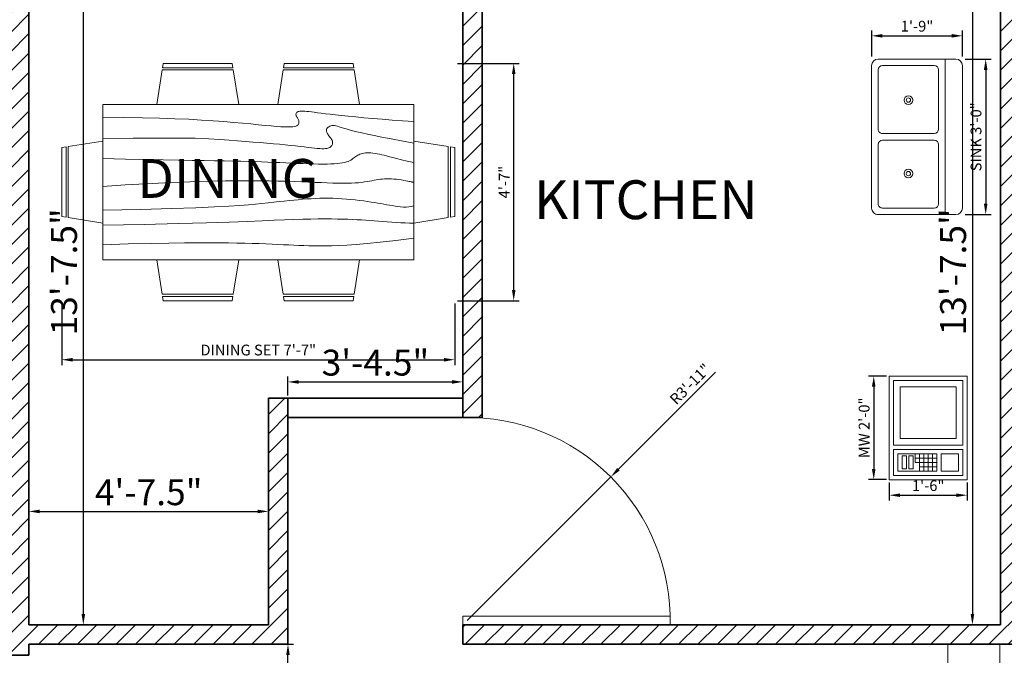
# Model space of a CAD drawing. Units: inches. Extents: x 4740 to 5323, y 7115 to 7713.
# Tile 4 of 6: x 4980 to 5208, y 7420 to 7567. Entities that reach past the tile are written whole.
import ezdxf

# ---------------------------------------------------------------- set-up
doc = ezdxf.new("R2010")
doc.units = ezdxf.units.IN
for name, color, linetype, lineweight in [('A-ANNO-DIMS', 2, 'Continuous', 18), ('A-AREA-IDEN', 7, 'Continuous', 25), ('A-DOOR', 4, 'Continuous', 18), ('A-EQPM', 8, 'Continuous', 18), ('A-FLOR-FIXT', 9, 'Continuous', 18), ('A-FLOR-STRS', 7, 'Continuous', 18), ('A-FURN', 8, 'Continuous', 18), ('A-WALL', 7, 'Continuous', 35)]:
    doc.layers.add(name, color=color, linetype=linetype, lineweight=lineweight)
doc.layers.add('A-WALL-PATT', color=152, linetype='Continuous', lineweight=13, true_color=0x2776bb)
doc.styles.get("Standard").update_dxf_attribs({"font": 'arial.ttf'})
doc.dimstyles.new('ISO-25', dxfattribs={"dimtxt": 2.5, "dimasz": 2.5, "dimexe": 1.25, "dimexo": 0.625, "dimtad": 1, "dimlunit": 3, "dimtxsty": 'Standard', "dimcen": 2.5, "dimadec": 0, "dimazin": 0, "dimtfac": 1, "dimtmove": 0, "dimatfit": 3, "dimfxl": 1, "dimarcsym": 0})

# ---------------------------------------------------------------- blocks, each defined once
blk = doc.blocks.new('*D22')
at = {"layer": 'A-ANNO-DIMS', "color": 0, "lineweight": -2, "transparency": 16777216}
for p, q in [((5206.33, 7590.36), (5199.17, 7590.36)), ((5200.42, 7587.86), (5200.42, 7429.36)), ((5206.33, 7426.86), (5199.17, 7426.86))]:
    blk.add_line(p, q, dxfattribs=at)
at = {"layer": 'A-ANNO-DIMS', "color": 0, "transparency": 16777216}
for points in [[(5200, 7587.86), (5200.84, 7587.86), (5200.42, 7590.36)], [(5200, 7429.36), (5200.84, 7429.36), (5200.42, 7426.86)]]:
    blk.add_solid(points, dxfattribs=at)
at = {"layer": 'Defpoints', "color": 0, "transparency": 16777216}
for p in [(5206.96, 7590.36), (5200.42, 7426.86), (5206.96, 7426.86)]:
    blk.add_point(p, dxfattribs=at)
at = {"layer": 'A-ANNO-DIMS', "color": 0, "transparency": 16777216, "insert": (5196.73, 7508.61), "char_height": 6, "attachment_point": 5, "rotation": 90}
blk.add_mtext('13\'-7.5"', dxfattribs=at)
blk = doc.blocks.new('*D29')
at = {"layer": 'A-ANNO-DIMS', "color": 0, "lineweight": -2, "transparency": 16777216}
for p, q in [((5012.58, 7422.36), (5043.21, 7422.36)), ((5041.96, 7303.66), (5041.96, 7419.86)), ((5026.08, 7301.16), (5043.21, 7301.16))]:
    blk.add_line(p, q, dxfattribs=at)
at = {"layer": 'A-ANNO-DIMS', "color": 0, "transparency": 16777216}
for points in [[(5041.54, 7419.86), (5042.38, 7419.86), (5041.96, 7422.36)], [(5041.54, 7303.66), (5042.38, 7303.66), (5041.96, 7301.16)]]:
    blk.add_solid(points, dxfattribs=at)
at = {"layer": 'Defpoints', "color": 0, "transparency": 16777216}
for p in [(5011.96, 7422.36), (5041.96, 7422.36), (5025.46, 7301.16)]:
    blk.add_point(p, dxfattribs=at)
at = {"layer": 'A-ANNO-DIMS', "color": 0, "transparency": 16777216, "insert": (5038.27, 7361.76), "char_height": 6, "attachment_point": 5, "rotation": 90}
blk.add_mtext('10\'-1.2"', dxfattribs=at)
blk = doc.blocks.new('*D30')
at = {"layer": 'A-ANNO-DIMS', "color": 0, "lineweight": -2, "transparency": 16777216}
for p, q in [((4981.96, 7427.48), (4981.96, 7454.36)), ((5037.46, 7427.48), (5037.46, 7454.36)), ((4984.46, 7453.11), (5034.96, 7453.11))]:
    blk.add_line(p, q, dxfattribs=at)
at = {"layer": 'A-ANNO-DIMS', "color": 0, "transparency": 16777216}
for points in [[(4984.46, 7453.52), (4984.46, 7452.69), (4981.96, 7453.11)], [(5034.96, 7453.52), (5034.96, 7452.69), (5037.46, 7453.11)]]:
    blk.add_solid(points, dxfattribs=at)
at = {"layer": 'Defpoints', "color": 0, "transparency": 16777216}
for p in [(5037.46, 7453.11), (4981.96, 7426.86), (5037.46, 7426.86)]:
    blk.add_point(p, dxfattribs=at)
at = {"layer": 'A-ANNO-DIMS', "color": 0, "transparency": 16777216, "insert": (5009.71, 7456.78), "char_height": 6, "attachment_point": 5}
blk.add_mtext('4\'-7.5"', dxfattribs=at)
blk = doc.blocks.new('*D31')
at = {"layer": 'A-ANNO-DIMS', "color": 0, "lineweight": -2, "transparency": 16777216}
for p, q in [((5041.96, 7479.98), (5041.96, 7484.36)), ((5082.46, 7479.98), (5082.46, 7484.36)), ((5044.46, 7483.11), (5079.96, 7483.11))]:
    blk.add_line(p, q, dxfattribs=at)
at = {"layer": 'A-ANNO-DIMS', "color": 0, "transparency": 16777216}
for points in [[(5044.46, 7483.52), (5044.46, 7482.69), (5041.96, 7483.11)], [(5079.96, 7483.52), (5079.96, 7482.69), (5082.46, 7483.11)]]:
    blk.add_solid(points, dxfattribs=at)
at = {"layer": 'Defpoints', "color": 0, "transparency": 16777216}
for p in [(5082.46, 7483.11), (5041.96, 7479.36), (5082.46, 7479.36)]:
    blk.add_point(p, dxfattribs=at)
at = {"layer": 'A-ANNO-DIMS', "color": 0, "transparency": 16777216, "insert": (5062.21, 7486.8), "char_height": 6, "attachment_point": 5}
blk.add_mtext('3\'-4.5"', dxfattribs=at)
blk = doc.blocks.new('*D32')
at = {"layer": 'A-ANNO-DIMS', "color": 0, "lineweight": -2, "transparency": 16777216}
for p, q in [((4982.58, 7590.36), (4995.83, 7590.36)), ((4994.58, 7587.86), (4994.58, 7429.36)), ((4982.58, 7426.86), (4995.83, 7426.86))]:
    blk.add_line(p, q, dxfattribs=at)
at = {"layer": 'A-ANNO-DIMS', "color": 0, "transparency": 16777216}
for points in [[(4994.17, 7587.86), (4995, 7587.86), (4994.58, 7590.36)], [(4994.17, 7429.36), (4995, 7429.36), (4994.58, 7426.86)]]:
    blk.add_solid(points, dxfattribs=at)
at = {"layer": 'Defpoints', "color": 0, "transparency": 16777216}
for p in [(4981.96, 7590.36), (4981.96, 7426.86), (4994.58, 7426.86)]:
    blk.add_point(p, dxfattribs=at)
at = {"layer": 'A-ANNO-DIMS', "color": 0, "transparency": 16777216, "insert": (4990.89, 7508.61), "char_height": 6, "attachment_point": 5, "rotation": 90}
blk.add_mtext('13\'-7.5"', dxfattribs=at)
blk = doc.blocks.new('Sink-double - 36 in top')
for p, q in [((-18, -4), (18, -4)), ((-0.75, -18.5), (-0.75, -6.5)), ((0.75, -6.5), (0.75, -18.5))]:
    blk.add_line(p, q)
for points in [[(-16.5, 0), (16.5, 0)], [(-18, -19.5), (-18, -1.5)], [(18, -1.5), (18, -19.5)], [(-16.5, -18.5), (-16.5, -6.5)], [(-15.5, -5.5), (-1.75, -5.5)], [(1.75, -5.5), (15.5, -5.5)], [(16.5, -6.5), (16.5, -18.5)], [(-1.75, -19.5), (-15.5, -19.5)], [(15.5, -19.5), (1.75, -19.5)], [(16.5, -21), (-16.5, -21)]]:
    blk.add_lwpolyline(points)
for centre, radius in [((-8.5, -12.5), 1), ((-8.5, -12.5), 0.5), ((8.5, -12.5), 1), ((8.5, -12.5), 0.5)]:
    blk.add_circle(centre, radius)
for centre, radius, start, end in [((-16.5, -1.5), 1.5, 90, 180), ((16.5, -1.5), 1.5, 0, 90), ((-15.5, -6.5), 1, 90, 180), ((-1.75, -6.5), 1, 0, 90), ((1.75, -6.5), 1, 90, 180), ((15.5, -6.5), 1, 0, 90), ((-16.5, -19.5), 1.5, 180, 270), ((-15.5, -18.5), 1, 180, 270), ((-1.75, -18.5), 1, 270, 0), ((1.75, -18.5), 1, 180, 270), ((15.5, -18.5), 1, 270, 0), ((16.5, -19.5), 1.5, 270, 0)]:
    blk.add_arc(centre, radius, start, end)
blk = doc.blocks.new('Microwave')
for p, q in [((18, 10), (22, 10)), ((19, 7), (19, 11)), ((20, 11), (20, 7)), ((21, 7), (21, 11)), ((22, 9), (18, 9)), ((18, 8), (22, 8)), ((22, 7), (18, 7)), ((19, 6), (19, 7)), ((20, 7), (20, 6)), ((20, 6), (18, 6))]:
    blk.add_line(p, q)
for points in [[(0, 0), (0, 18), (24, 18), (24, 0)], [(1, 1), (1, 17), (16, 17), (16, 1)], [(17, 1), (17, 17), (23, 17), (23, 1)], [(18, 12), (18, 16), (22, 16), (22, 12)], [(2.5, 2.5), (2.5, 15.5), (14.5, 15.5), (14.5, 2.5)], [(18, 2), (18, 11), (22, 11), (22, 2)], [(18.5, 4.5), (18.5, 5.5), (21.5, 5.5), (21.5, 4.5)], [(18.5, 3), (18.5, 4), (21.5, 4), (21.5, 3)]]:
    blk.add_lwpolyline(points, close=True)
blk = doc.blocks.new('Dining Set - 36 x 72 in.')
for p, q in [((-22, 27.5), (-22.1562, 26.50042)), ((-22, 27.5), (-6, 27.5)), ((-5.8437, 26.49966), (-6, 27.5)), ((6, 27.5), (5.8438, 26.50042)), ((6, 27.5), (22, 27.5)), ((22.1563, 26.49966), (22, 27.5)), ((-22.2343, 26.00059), (-23.4847, 17.99762)), ((-22.2304, 26), (-5.7608, 26)), ((-5.8416, 26.5), (-22.1534, 26.5)), ((-4.5152, 17.99762), (-5.7655, 25.99926)), ((5.7657, 26.00059), (4.5153, 17.99762)), ((5.7696, 26), (22.2392, 26)), ((22.1584, 26.5), (5.8466, 26.5)), ((23.4848, 17.99762), (22.2345, 25.99926)), ((36, 18), (-36, 18)), ((-36, 18), (-36, -18)), ((36, -18), (36, 18)), ((-44.0006, 8.23428), (-35.9976, 9.48474)), ((44.0006, 8.23428), (35.9976, 9.48474)), ((-45.5, 8), (-44.5004, 8.15617)), ((-45.5, 8), (-45.5, -8)), ((-44.5, -8.15843), (-44.5, 8.15338)), ((-44, 8.23041), (-44, -8.23915)), ((44, 8.23041), (44, -8.23915)), ((44.5, -8.15843), (44.5, 8.15338)), ((45.5, 8), (44.5005, 8.15617)), ((45.5, 8), (45.5, -8)), ((-44.4997, -8.15631), (-45.5, -8)), ((-35.9976, -9.48476), (-43.9993, -8.2345)), ((35.9976, -9.48476), (43.9993, -8.2345)), ((44.4997, -8.15631), (45.5, -8)), ((-36, -18), (36, -18)), ((-22.2343, -26.0006), (-23.4847, -17.99762)), ((-4.5152, -17.99762), (-5.7655, -25.99928)), ((5.7657, -26.0006), (4.5153, -17.99762)), ((23.4848, -17.99762), (22.2345, -25.99928)), ((-22.2304, -26), (-5.7608, -26)), ((-22, -27.5), (-22.1562, -26.50044)), ((-5.8416, -26.5), (-22.1534, -26.5)), ((-5.8437, -26.49967), (-6, -27.5)), ((5.7696, -26), (22.2392, -26)), ((6, -27.5), (5.8438, -26.50044)), ((22.1584, -26.5), (5.8466, -26.5)), ((22.1563, -26.49967), (22, -27.5)), ((-22, -27.5), (-6, -27.5)), ((6, -27.5), (22, -27.5))]:
    blk.add_line(p, q)
for points in [[(-36, 15), (-31.1772, 14.97754), (-26.8079, 14.91406), (-22.8538, 14.81543), (-19.276, 14.6875), (-16.0362, 14.53613), (-13.0957, 14.36718), (-10.4159, 14.18652), (-7.9583, 14), (-5.6904, 13.81315), (-3.6035, 13.63021), (-1.6954, 13.45508), (0.0365, 13.29166), (1.5945, 13.14388), (2.9811, 13.01562), (4.1988, 12.9108), (5.25, 12.83333), (6.1393, 12.78613), (6.8802, 12.76823), (7.4883, 12.77767), (7.9792, 12.8125), (8.3685, 12.87077), (8.6719, 12.95052), (8.9049, 13.0498), (9.0833, 13.16666), (9.2205, 13.29899), (9.3216, 13.44401), (9.3895, 13.59879), (9.4271, 13.76041), (9.4373, 13.92594), (9.4232, 14.09245), (9.3875, 14.257), (9.3333, 14.41666), (9.2638, 14.56917), (9.1836, 14.71484), (9.0975, 14.85465), (9.0104, 14.98958), (8.9272, 15.1206), (8.8529, 15.2487), (8.7922, 15.37483), (8.75, 15.5), (8.7305, 15.62467), (8.7344, 15.74739), (8.7617, 15.86621), (8.8125, 15.97916), (8.8867, 16.08431), (8.9844, 16.17968), (9.1055, 16.26334), (9.25, 16.33333), (9.4189, 16.38802), (9.6172, 16.42708), (9.8506, 16.45052), (10.125, 16.45833), (10.4463, 16.45052), (10.8203, 16.42708), (11.2529, 16.38802), (11.75, 16.33333), (12.3184, 16.26318), (12.9694, 16.17838), (13.7151, 16.07991), (14.5677, 15.96875), (15.5395, 15.84586), (16.6426, 15.71224), (17.8893, 15.56884), (19.2917, 15.41666), (20.859, 15.25667), (22.5879, 15.08984), (24.4721, 14.91715), (26.5052, 14.73958), (28.6809, 14.5581), (30.9929, 14.3737), (33.4347, 14.18733), (36, 14)], [(-36, 10), (-28.9766, 10.14274), (-23.1725, 10.20442), (-18.4241, 10.19775), (-14.5677, 10.13541), (-11.4399, 10.03011), (-8.877, 9.89453), (-6.7154, 9.74137), (-4.7917, 9.58333), (-2.9698, 9.43082), (-1.2246, 9.28515), (0.4415, 9.14534), (2.026, 9.01041), (3.5266, 8.87939), (4.9408, 8.7513), (6.266, 8.62516), (7.5, 8.5), (8.6411, 8.37549), (9.6914, 8.2539), (10.6538, 8.13818), (11.5312, 8.03125), (12.3267, 7.93603), (13.043, 7.85547), (13.6831, 7.79248), (14.25, 7.75), (14.7471, 7.7303), (15.1797, 7.73307), (15.5537, 7.75732), (15.875, 7.80208), (16.1494, 7.86637), (16.3828, 7.94922), (16.5811, 8.04964), (16.75, 8.16666), (16.8944, 8.29915), (17.0143, 8.44531), (17.1089, 8.60319), (17.1771, 8.77083), (17.218, 8.94629), (17.2305, 9.1276), (17.2137, 9.31282), (17.1667, 9.5), (17.0895, 9.6875), (16.987, 9.875), (16.8649, 10.0625), (16.7292, 10.25), (16.5856, 10.4375), (16.4401, 10.625), (16.2985, 10.8125), (16.1667, 11), (16.05, 11.18733), (15.9518, 11.3737), (15.8752, 11.5581), (15.8229, 11.73958), (15.798, 11.91715), (15.8034, 12.08984), (15.842, 12.25667), (15.9167, 12.41666), (16.0295, 12.56836), (16.1784, 12.70833), (16.3605, 12.83268), (16.5729, 12.9375), (16.8127, 13.01888), (17.0768, 13.07291), (17.3625, 13.0957), (17.6667, 13.08333), (17.9894, 13.03312), (18.3418, 12.94726), (18.7382, 12.82918), (19.1927, 12.68229), (19.7195, 12.51001), (20.3327, 12.31575), (21.0465, 12.10294), (21.875, 11.875), (22.8357, 11.63354), (23.959, 11.37304), (25.2786, 11.08618), (26.8282, 10.76562), (28.6414, 10.40405), (30.752, 9.99414), (33.1936, 9.52856), (36, 9)], [(-36, 5.5), (-30.7157, 5.3348), (-26.069, 5.20963), (-21.9946, 5.11767), (-18.4271, 5.05208), (-15.3009, 5.00602), (-12.5508, 4.97265), (-10.1112, 4.94515), (-7.9167, 4.91666), (-5.909, 4.88167), (-4.0586, 4.83984), (-2.3429, 4.79215), (-0.7396, 4.73958), (0.7739, 4.6831), (2.22, 4.6237), (3.6213, 4.56233), (5, 4.5), (6.373, 4.43782), (7.7344, 4.3776), (9.0723, 4.32129), (10.375, 4.27083), (11.6309, 4.22819), (12.8281, 4.19531), (13.9551, 4.17415), (15, 4.16666), (15.954, 4.17448), (16.819, 4.19791), (17.6001, 4.23698), (18.3021, 4.29166), (18.9299, 4.36198), (19.4883, 4.44791), (19.9823, 4.54948), (20.4167, 4.66666), (20.7969, 4.79899), (21.1302, 4.94401), (21.4245, 5.09879), (21.6875, 5.26041), (21.9271, 5.42594), (22.1511, 5.59245), (22.3672, 5.757), (22.5834, 5.91666), (22.8065, 6.06868), (23.0404, 6.21093), (23.2879, 6.34147), (23.5521, 6.45833), (23.8358, 6.55957), (24.142, 6.64323), (24.4735, 6.70735), (24.8334, 6.75), (25.2235, 6.76969), (25.642, 6.76692), (26.0858, 6.74267), (26.5521, 6.69791), (27.0379, 6.63362), (27.5404, 6.55078), (28.0565, 6.45036), (28.5834, 6.33333), (29.1242, 6.19987), (29.7071, 6.04687), (30.3661, 5.87044), (31.1354, 5.66666), (32.0493, 5.43164), (33.142, 5.16146), (34.4475, 4.85221), (36, 4.5)], [(-36, -1), (-30.7915, -0.6591), (-26.0195, -0.38216), (-21.6519, -0.16284), (-17.6563, 0.00521), (-14.0005, 0.12833), (-10.6523, 0.21289), (-7.5796, 0.26522), (-4.75, 0.29166), (-2.134, 0.29793), (0.2878, 0.28711), (2.5317, 0.26163), (4.6146, 0.22396), (6.5529, 0.17651), (8.3633, 0.12174), (10.0623, 0.06209), (11.6667, 0), (13.1899, -0.06201), (14.6341, -0.1211), (15.9982, -0.17432), (17.2813, -0.21875), (18.4823, -0.25147), (19.6003, -0.26953), (20.6343, -0.27002), (21.5834, -0.25), (22.4481, -0.20768), (23.2357, -0.14584), (23.9549, -0.06836), (24.6146, 0.02083), (25.2235, 0.11784), (25.7904, 0.21875), (26.3241, 0.31966), (26.8334, 0.41666), (27.3265, 0.50618), (27.8099, 0.58593), (28.2894, 0.65397), (28.7709, 0.70833), (29.2601, 0.74707), (29.763, 0.76823), (30.2855, 0.76985), (30.8334, 0.75), (31.4088, 0.70784), (31.9994, 0.64713), (32.589, 0.57275), (33.1615, 0.48958), (33.7008, 0.4025), (34.1908, 0.3164), (34.6153, 0.23616), (34.9584, 0.16666), (35.2099, 0.11165), (35.3848, 0.07031), (35.504, 0.04069), (35.5886, 0.02083), (35.6594, 0.00879), (35.7377, 0.0026), (35.8442, 0.00032), (36, 0)], [(-36, -6.5), (-27.1843, -6.31267), (-20.084, -6.1263), (-14.469, -5.9419), (-10.1094, -5.76042), (-6.7752, -5.58285), (-4.2363, -5.41016), (-2.2629, -5.24333), (-0.625, -5.08334), (0.8708, -4.93099), (2.2715, -4.78646), (3.5872, -4.64974), (4.8281, -4.52084), (6.0046, -4.39974), (7.127, -4.28646), (8.2053, -4.18099), (9.25, -4.08334), (10.2705, -3.99382), (11.2734, -3.91407), (12.2647, -3.84603), (13.25, -3.79167), (14.2354, -3.75293), (15.2266, -3.73177), (16.2295, -3.73015), (17.25, -3.75), (18.2912, -3.79248), (19.3451, -3.85547), (20.4009, -3.93604), (21.4479, -4.03125), (22.4754, -4.13819), (23.4727, -4.25391), (24.4289, -4.37549), (25.3334, -4.5), (26.1785, -4.62492), (26.9694, -4.74935), (27.7145, -4.87281), (28.4219, -4.99479), (29.1, -5.11483), (29.7572, -5.23242), (30.4016, -5.34709), (31.0417, -5.45834), (31.6837, -5.56437), (32.3262, -5.65821), (32.9658, -5.73153), (33.599, -5.77604), (34.2224, -5.78345), (34.8327, -5.74545), (35.4264, -5.65373), (36, -5.5)], [(-36, -10), (-26.4022, -9.81299), (-18.4675, -9.62891), (-11.9839, -9.45069), (-6.7396, -9.28125), (-2.5226, -9.12354), (0.8789, -8.98047), (3.6769, -8.85498), (6.0833, -8.75), (8.2767, -8.66765), (10.3021, -8.60677), (12.1712, -8.56543), (13.8958, -8.54167), (15.4876, -8.53353), (16.9583, -8.53907), (18.3197, -8.55632), (19.5834, -8.58334), (20.7616, -8.61841), (21.8685, -8.66081), (22.9188, -8.71004), (23.9271, -8.76563), (24.9081, -8.82707), (25.8763, -8.89388), (26.8465, -8.96558), (27.8334, -9.04167), (28.8474, -9.12118), (29.8828, -9.20117), (30.93, -9.27824), (31.9792, -9.34896), (33.0205, -9.40991), (34.0443, -9.45768), (35.0407, -9.48885), (36, -9.5)], [(-36, -14.5), (-30.0881, -14.33513), (-25.0332, -14.21224), (-20.7312, -14.12647), (-17.0781, -14.07292), (-13.97, -14.04671), (-11.3027, -14.04297), (-8.9724, -14.05681), (-6.875, -14.08334), (-4.9224, -14.11833), (-3.0905, -14.16016), (-1.3709, -14.20785), (0.2448, -14.26042), (1.7647, -14.3169), (3.1973, -14.3763), (4.5507, -14.43767), (5.8333, -14.5), (7.0554, -14.5621), (8.235, -14.62175), (9.3922, -14.67652), (10.5469, -14.72396), (11.7192, -14.76164), (12.929, -14.78711), (14.1965, -14.79794), (15.5417, -14.79167), (16.9933, -14.76424), (18.6152, -14.70508), (20.4804, -14.60197), (22.6615, -14.44271), (25.2312, -14.21509), (28.2624, -13.9069), (31.8277, -13.50594), (36, -13)]]:
    blk.add_lwpolyline(points)
blk = doc.blocks.new('*D36')
at = {"layer": 'A-ANNO-DIMS', "color": 0, "lineweight": -2, "transparency": 16777216}
for p, q in [((5078.58, 7675.86), (5323.05, 7675.86)), ((5321.8, 7673.36), (5321.8, 7150.66)), ((5077.56, 7148.16), (5323.05, 7148.16))]:
    blk.add_line(p, q, dxfattribs=at)
at = {"layer": 'A-ANNO-DIMS', "color": 0, "transparency": 16777216}
for points in [[(5321.38, 7673.36), (5322.22, 7673.36), (5321.8, 7675.86)], [(5321.38, 7150.66), (5322.22, 7150.66), (5321.8, 7148.16)]]:
    blk.add_solid(points, dxfattribs=at)
at = {"layer": 'Defpoints', "color": 0, "transparency": 16777216}
for p in [(5077.96, 7675.86), (5076.93, 7148.16), (5321.8, 7148.16)]:
    blk.add_point(p, dxfattribs=at)
at = {"layer": 'A-ANNO-DIMS', "color": 0, "transparency": 16777216, "insert": (5318.11, 7412.01), "char_height": 6, "attachment_point": 5, "rotation": 90}
blk.add_mtext('43\'-11.7"', dxfattribs=at)
blk = doc.blocks.new('*D60')
at = {"layer": 'A-ANNO-DIMS', "color": 0, "lineweight": -2, "transparency": 16777216}
for p, q in [((5198.72, 7557.88), (5204.75, 7557.88)), ((5203.5, 7555.38), (5203.5, 7524.38)), ((5198.72, 7521.88), (5204.75, 7521.88))]:
    blk.add_line(p, q, dxfattribs=at)
at = {"layer": 'A-ANNO-DIMS', "color": 0, "transparency": 16777216}
for points in [[(5203.08, 7555.38), (5203.91, 7555.38), (5203.5, 7557.88)], [(5203.08, 7524.38), (5203.91, 7524.38), (5203.5, 7521.88)]]:
    blk.add_solid(points, dxfattribs=at)
at = {"layer": 'Defpoints', "color": 0, "transparency": 16777216}
for p in [(5198.1, 7557.88), (5198.1, 7521.88), (5203.5, 7521.88)]:
    blk.add_point(p, dxfattribs=at)
at = {"layer": 'A-ANNO-DIMS', "color": 0, "transparency": 16777216, "insert": (5201.58, 7539.88), "char_height": 2.5, "attachment_point": 5, "rotation": 90}
blk.add_mtext('SINK 3\'-0"', dxfattribs=at)
blk = doc.blocks.new('*D61')
at = {"layer": 'A-ANNO-DIMS', "color": 0, "lineweight": -2, "transparency": 16777216}
for p, q in [((5177.1, 7558.5), (5177.1, 7564.53)), ((5198.1, 7558.5), (5198.1, 7564.53)), ((5179.6, 7563.28), (5195.6, 7563.28))]:
    blk.add_line(p, q, dxfattribs=at)
at = {"layer": 'A-ANNO-DIMS', "color": 0, "transparency": 16777216}
for points in [[(5179.6, 7563.7), (5179.6, 7562.86), (5177.1, 7563.28)], [(5195.6, 7563.7), (5195.6, 7562.86), (5198.1, 7563.28)]]:
    blk.add_solid(points, dxfattribs=at)
at = {"layer": 'Defpoints', "color": 0, "transparency": 16777216}
for p in [(5198.1, 7563.28), (5177.1, 7557.88), (5198.1, 7557.88)]:
    blk.add_point(p, dxfattribs=at)
at = {"layer": 'A-ANNO-DIMS', "color": 0, "transparency": 16777216, "insert": (5187.6, 7565.18), "char_height": 2.5, "attachment_point": 5}
blk.add_mtext('1\'-9"', dxfattribs=at)
blk = doc.blocks.new('*D62')
at = {"layer": 'A-ANNO-DIMS', "color": 0, "lineweight": -2, "transparency": 16777216}
for p, q in [((5180.55, 7484.47), (5176.33, 7484.47)), ((5177.58, 7481.97), (5177.58, 7462.97)), ((5180.55, 7460.47), (5176.33, 7460.47))]:
    blk.add_line(p, q, dxfattribs=at)
at = {"layer": 'A-ANNO-DIMS', "color": 0, "transparency": 16777216}
for points in [[(5177.16, 7481.97), (5177.99, 7481.97), (5177.58, 7484.47)], [(5177.16, 7462.97), (5177.99, 7462.97), (5177.58, 7460.47)]]:
    blk.add_solid(points, dxfattribs=at)
at = {"layer": 'Defpoints', "color": 0, "transparency": 16777216}
for p in [(5181.18, 7484.47), (5177.58, 7460.47), (5181.18, 7460.47)]:
    blk.add_point(p, dxfattribs=at)
at = {"layer": 'A-ANNO-DIMS', "color": 0, "transparency": 16777216, "insert": (5175.68, 7472.47), "char_height": 2.5, "attachment_point": 5, "rotation": 90}
blk.add_mtext('MW 2\'-0"', dxfattribs=at)
blk = doc.blocks.new('*D63')
at = {"layer": 'A-ANNO-DIMS', "color": 0, "lineweight": -2, "transparency": 16777216}
for p, q in [((5181.18, 7459.84), (5181.18, 7455.62)), ((5199.18, 7459.84), (5199.18, 7455.62)), ((5183.68, 7456.87), (5196.68, 7456.87))]:
    blk.add_line(p, q, dxfattribs=at)
at = {"layer": 'A-ANNO-DIMS', "color": 0, "transparency": 16777216}
for points in [[(5183.68, 7457.28), (5183.68, 7456.45), (5181.18, 7456.87)], [(5196.68, 7457.28), (5196.68, 7456.45), (5199.18, 7456.87)]]:
    blk.add_solid(points, dxfattribs=at)
at = {"layer": 'Defpoints', "color": 0, "transparency": 16777216}
for p in [(5181.18, 7460.47), (5199.18, 7460.47), (5199.18, 7456.87)]:
    blk.add_point(p, dxfattribs=at)
at = {"layer": 'A-ANNO-DIMS', "color": 0, "transparency": 16777216, "insert": (5190.18, 7458.77), "char_height": 2.5, "attachment_point": 5}
blk.add_mtext('1\'-6"', dxfattribs=at)
blk = doc.blocks.new('*D64')
at = {"layer": 'A-ANNO-DIMS', "color": 0, "lineweight": -2, "transparency": 16777216}
for p, q in [((4989.58, 7501.27), (4989.58, 7487)), ((5080.58, 7501.27), (5080.58, 7487)), ((4992.08, 7488.25), (5078.08, 7488.25))]:
    blk.add_line(p, q, dxfattribs=at)
at = {"layer": 'A-ANNO-DIMS', "color": 0, "transparency": 16777216}
for points in [[(4992.08, 7488.66), (4992.08, 7487.83), (4989.58, 7488.25)], [(5078.08, 7488.66), (5078.08, 7487.83), (5080.58, 7488.25)]]:
    blk.add_solid(points, dxfattribs=at)
at = {"layer": 'Defpoints', "color": 0, "transparency": 16777216}
for p in [(4989.58, 7501.9), (5080.58, 7501.9), (5080.58, 7488.25)]:
    blk.add_point(p, dxfattribs=at)
at = {"layer": 'A-ANNO-DIMS', "color": 0, "transparency": 16777216, "insert": (5035.08, 7490.17), "char_height": 2.5, "attachment_point": 5}
blk.add_mtext('DINING SET 7\'-7"', dxfattribs=at)
blk = doc.blocks.new('*D65')
at = {"layer": 'A-ANNO-DIMS', "color": 0, "lineweight": -2, "transparency": 16777216}
for p, q in [((5081.2, 7556.9), (5095.48, 7556.9)), ((5094.23, 7504.4), (5094.23, 7554.4)), ((5081.2, 7501.9), (5095.48, 7501.9))]:
    blk.add_line(p, q, dxfattribs=at)
at = {"layer": 'A-ANNO-DIMS', "color": 0, "transparency": 16777216}
for points in [[(5093.81, 7554.4), (5094.64, 7554.4), (5094.23, 7556.9)], [(5093.81, 7504.4), (5094.64, 7504.4), (5094.23, 7501.9)]]:
    blk.add_solid(points, dxfattribs=at)
at = {"layer": 'Defpoints', "color": 0, "transparency": 16777216}
for p in [(5080.58, 7556.9), (5094.23, 7556.9), (5080.58, 7501.9)]:
    blk.add_point(p, dxfattribs=at)
at = {"layer": 'A-ANNO-DIMS', "color": 0, "transparency": 16777216, "insert": (5092.35, 7529.4), "char_height": 2.5, "attachment_point": 5, "rotation": 90}
blk.add_mtext('4\'-7"', dxfattribs=at)
blk = doc.blocks.new('*D81')
at = {"layer": 'A-ANNO-DIMS', "color": 0, "lineweight": -2, "transparency": 16777216}
for p, q in [((4776.46, 7632.98), (4776.46, 7708.41)), ((5264.46, 7707.16), (4778.96, 7707.16)), ((5266.96, 7422.98), (5266.96, 7708.41))]:
    blk.add_line(p, q, dxfattribs=at)
at = {"layer": 'A-ANNO-DIMS', "color": 0, "transparency": 16777216}
for points in [[(4778.96, 7707.57), (4778.96, 7706.74), (4776.46, 7707.16)], [(5264.46, 7707.57), (5264.46, 7706.74), (5266.96, 7707.16)]]:
    blk.add_solid(points, dxfattribs=at)
at = {"layer": 'Defpoints', "color": 0, "transparency": 16777216}
for p in [(4776.46, 7707.16), (4776.46, 7632.36), (5266.96, 7422.36)]:
    blk.add_point(p, dxfattribs=at)
at = {"layer": 'A-ANNO-DIMS', "color": 0, "transparency": 16777216, "insert": (5021.71, 7709.07), "char_height": 2.5, "attachment_point": 5}
blk.add_mtext('40\'-10 1/2"', dxfattribs=at)
blk = doc.blocks.new('*D88')
at = {"layer": 'A-ANNO-DIMS', "color": 0, "lineweight": -2, "transparency": 16777216}
for p, q in [((5140.97, 7485.37), (5118.47, 7462.87)), ((5083.46, 7427.86), (5116.7, 7461.1))]:
    blk.add_line(p, q, dxfattribs=at)
at = {"layer": 'A-ANNO-DIMS', "color": 0, "transparency": 16777216}
blk.add_solid([(5118.17, 7463.16), (5118.76, 7462.57), (5116.7, 7461.1)], dxfattribs=at)
at = {"layer": 'Defpoints', "color": 0, "transparency": 16777216}
for p in [(5116.7, 7461.1), (5083.46, 7427.86)]:
    blk.add_point(p, dxfattribs=at)
at = {"layer": 'A-ANNO-DIMS', "color": 0, "transparency": 16777216, "insert": (5135.3, 7482.39), "char_height": 2.5, "attachment_point": 5, "rotation": 44.9995}
blk.add_mtext('R3\'-11"', dxfattribs=at)
blk = doc.blocks.new('*D90')
at = {"layer": 'A-ANNO-DIMS', "color": 0, "lineweight": -2, "transparency": 16777216}
for p, q in [((4940.01, 7425.47), (4958.3, 7409.76)), ((4986.12, 7385.86), (4960.2, 7408.13))]:
    blk.add_line(p, q, dxfattribs=at)
at = {"layer": 'A-ANNO-DIMS', "color": 0, "transparency": 16777216}
blk.add_solid([(4958.57, 7410.07), (4958.03, 7409.44), (4960.2, 7408.13)], dxfattribs=at)
at = {"layer": 'Defpoints', "color": 0, "transparency": 16777216}
for p in [(4960.2, 7408.13), (4986.12, 7385.86)]:
    blk.add_point(p, dxfattribs=at)
at = {"layer": 'A-ANNO-DIMS', "color": 0, "transparency": 16777216, "insert": (4945.88, 7422.93), "char_height": 2.5, "attachment_point": 5, "rotation": 319.334}
blk.add_mtext('R2\'-10"', dxfattribs=at)

msp = doc.modelspace()

# ---------------------------------------------------------------- hatches: boundary and pattern name
at = {"layer": 'A-WALL-PATT'}
h = msp.add_hatch(dxfattribs=at)
h.set_pattern_fill('ANSI31', color=256)
h.paths.add_polyline_path([(4925.343, 7632.357), (4776.459, 7632.357), (4776.459, 7486.448), (4785.459, 7486.448), (4785.459, 7522.857), (4959.459, 7522.857), (4959.459, 7527.357), (4785.459, 7527.357), (4785.459, 7623.357), (4833.459, 7623.357), (4925.343, 7623.357)])
h.paths.add_polyline_path([(5010.258, 7599.357), (5004.258, 7599.357), (4986.459, 7599.357), (4986.459, 7623.357), (4986.459, 7632.357), (4977.459, 7632.357), (4949.343, 7632.357), (4949.343, 7623.357), (4977.459, 7623.357), (4977.459, 7599.357), (4977.459, 7594.857), (4977.459, 7590.357), (4977.459, 7524.857, -0.0293864), (4977.459, 7522.857), (4977.459, 7426.857), (4977.459, 7422.357), (4977.459, 7419.778), (4981.959, 7419.778), (4981.959, 7422.357), (5041.959, 7422.357), (5041.959, 7479.357), (5037.459, 7479.357), (5037.459, 7426.857), (4981.959, 7426.857), (4981.959, 7590.357), (5010.258, 7590.357)])
h.paths.add_polyline_path([(5086.959, 7666.857), (5206.959, 7666.857), (5206.959, 7646.624), (5215.959, 7646.624), (5215.959, 7675.857), (5077.959, 7675.857), (5077.959, 7599.357), (5046.258, 7599.357), (5046.258, 7590.357), (5082.459, 7590.357), (5082.459, 7474.857, -0.0106371), (5084.459, 7474.857), (5086.959, 7474.857)])
h.paths.add_polyline_path([(5215.959, 7610.624), (5206.959, 7610.624), (5206.959, 7594.857), (5104.959, 7594.857), (5104.959, 7592.357, -0.0293864), (5104.959, 7590.357), (5206.959, 7590.357), (5206.959, 7426.857), (5104.959, 7426.857), (5082.459, 7426.857), (5082.459, 7422.357), (5104.959, 7422.357), (5215.959, 7422.357), (5215.959, 7464.357), (5215.959, 7506.357)])
h.paths.add_polyline_path([(4881.459, 7375.857), (4977.459, 7375.857), (4977.459, 7296.657), (4981.959, 7296.657), (4981.959, 7384.857), (4951.959, 7384.857), (4785.459, 7384.857), (4785.459, 7438.448), (4776.459, 7438.448), (4776.459, 7375.857), (4872.459, 7375.857), (4872.459, 7337.044), (4881.459, 7337.044)])
h.paths.add_polyline_path([(4881.459, 7313.044), (4872.459, 7313.044), (4872.459, 7148.157), (4916.568, 7148.157), (4916.568, 7157.157), (4881.459, 7157.157), (4881.459, 7269.357), (4981.959, 7269.357), (4981.959, 7273.857), (4963.959, 7273.857), (4881.459, 7273.857)])
h.paths.add_polyline_path([(5029.959, 7296.657), (5116.509, 7296.657), (5116.509, 7299.157, -0.0121933), (5116.509, 7301.157), (5025.459, 7301.157), (5025.459, 7157.157), (4964.568, 7157.157), (4964.568, 7148.157), (5076.933, 7148.157), (5076.933, 7157.157), (5029.959, 7157.157)])
h.paths.add_polyline_path([(5182.959, 7203.442), (5173.959, 7203.442), (5173.959, 7157.157), (5124.933, 7157.157), (5124.933, 7148.157), (5182.959, 7148.157)])
h.paths.add_polyline_path([(5266.959, 7353.764), (5257.959, 7353.764), (5257.959, 7301.157), (5182.959, 7301.157), (5158.509, 7301.157), (5158.509, 7296.657), (5173.959, 7296.657), (5173.959, 7263.442), (5182.959, 7263.442), (5182.959, 7292.157), (5266.959, 7292.157)])
h.paths.add_polyline_path([(5266.959, 7422.357), (5257.959, 7422.357), (5257.959, 7377.764), (5266.959, 7377.764)])

# ---------------------------------------------------------------- linework, layer by layer
at = {"layer": 'A-DOOR'}
for p, q in [((5130.459, 7428.857), (5082.459, 7428.857)), ((5082.459, 7428.857), (5082.459, 7426.857)), ((5082.459, 7426.857), (5130.459, 7426.857)), ((5130.459, 7426.857), (5130.459, 7428.857))]:
    msp.add_line(p, q, dxfattribs=at)
msp.add_arc((5083.459, 7427.857), 47.011, 358.78112, 91.21888, dxfattribs=at)
at = {"layer": 'A-FLOR-STRS'}
for p, q in [((5194.734, 7301.157), (5194.734, 7422.357)), ((5206.734, 7301.157), (5206.734, 7422.357))]:
    msp.add_line(p, q, dxfattribs=at)
at = {"layer": 'A-WALL'}
for p, q in [((5086.959, 7666.857), (5086.959, 7474.857)), ((4981.959, 7590.357), (4981.959, 7426.857)), ((5082.459, 7590.357), (5082.459, 7474.857)), ((5206.959, 7590.357), (5206.959, 7426.857)), ((5037.459, 7479.357), (5037.459, 7426.857)), ((5037.459, 7479.357), (5082.459, 7479.357)), ((5041.959, 7479.357), (5041.959, 7422.357)), ((5041.959, 7474.857), (5086.959, 7474.857)), ((4981.959, 7426.857), (5037.459, 7426.857)), ((5082.459, 7426.857), (5104.959, 7426.857)), ((5104.959, 7426.857), (5082.459, 7426.857)), ((5082.459, 7426.857), (5082.459, 7422.357)), ((5104.959, 7426.857), (5206.959, 7426.857)), ((4981.959, 7422.357), (5041.959, 7422.357)), ((4981.959, 7419.778), (4981.959, 7422.357)), ((5082.459, 7422.357), (5104.959, 7422.357)), ((5104.959, 7422.357), (5215.959, 7422.357)), ((4977.459, 7419.778), (4981.959, 7419.778))]:
    msp.add_line(p, q, dxfattribs=at)

# ---------------------------------------------------------------- block references
at = {"layer": 'A-EQPM', "rotation": 270}
msp.add_blockref('Microwave', (5181.178, 7484.465), dxfattribs=at)
at = {"layer": 'A-FLOR-FIXT', "rotation": 270}
msp.add_blockref('Sink-double - 36 in top', (5198.095, 7539.88), dxfattribs=at)
at = {"layer": 'A-FURN'}
msp.add_blockref('Dining Set - 36 x 72 in.', (5035.076, 7529.398), dxfattribs=at)

# ---------------------------------------------------------------- texts
at = {"layer": 'A-AREA-IDEN', "char_height": 9, "attachment_point": 1}
for s, insert in [('{ DINING}', (5004.36, 7534.733)), ('{ KITCHEN}', (5096.166, 7529.812))]:
    msp.add_mtext_dynamic_manual_height_columns(s, width=75.84022, gutter_width=12.5, heights=[0], dxfattribs=dict(at, insert=insert))

# ---------------------------------------------------------------- dimensions: what is measured, and where the dimension line sits
at = {"layer": 'A-ANNO-DIMS'}
for base, p1, p2, override, picture, middle in [((4776.459, 7707.157), (5266.959, 7422.357), (4776.459, 7632.357), {"dimdec": 1, "dimlfac": 1, "dimrnd": 0, "dimzin": 1, "dimdsep": 46, "dimlunit": 4, "dimfrac": 2}, '*D81', (5021.709, 7709.074)), ((5198.095, 7563.28), (5177.095, 7557.88), (5198.095, 7557.88), {"dimdec": 1, "dimlfac": 1, "dimrnd": 0, "dimzin": 1, "dimdsep": 46, "dimlunit": 4, "dimfrac": 2}, '*D61', (5187.595, 7565.181)), ((5037.459, 7453.107), (4981.959, 7426.857), (5037.459, 7426.857), {"dimtxt": 6, "dimclrd": 0, "dimclre": 0, "dimclrt": 0}, '*D30', (5009.709, 7456.783)), ((5199.178, 7456.865), (5181.178, 7460.465), (5199.178, 7460.465), {"dimdec": 1, "dimlfac": 1, "dimrnd": 0, "dimzin": 1, "dimdsep": 46, "dimlunit": 4, "dimfrac": 2}, '*D63', (5190.178, 7458.767))]:
    dim = msp.add_linear_dim(base=base, p1=p1, p2=p2, dimstyle='ISO-25', override=override, dxfattribs=at)
    dim.commit()
    dim.dimension.update_dxf_attribs({"geometry": picture, "text_midpoint": middle})
for base, p1, p2, override, picture, middle in [((5321.801, 7148.157), (5077.959, 7675.857), (5076.933, 7148.157), {"dimtxt": 6, "dimclrd": 0, "dimclre": 0, "dimclrt": 0}, '*D36', (5318.111, 7412.007)), ((4994.583, 7426.857), (4981.959, 7590.357), (4981.959, 7426.857), {"dimtxt": 6, "dimclrd": 0, "dimclre": 0, "dimclrt": 0}, '*D32', (4990.893, 7508.607)), ((5094.226, 7556.898), (5080.576, 7501.898), (5080.576, 7556.898), {"dimdec": 1, "dimlfac": 1, "dimrnd": 0, "dimzin": 1, "dimdsep": 46, "dimlunit": 4, "dimfrac": 2}, '*D65', (5092.351, 7529.398)), ((5041.959, 7422.357), (5025.459, 7301.157), (5011.959, 7422.357), {"dimtxt": 6, "dimclrd": 0, "dimclre": 0, "dimclrt": 0}, '*D29', (5038.271, 7361.757))]:
    dim = msp.add_linear_dim(base=base, p1=p1, p2=p2, angle=90, dimstyle='ISO-25', override=override, dxfattribs=at)
    dim.commit()
    dim.dimension.update_dxf_attribs({"geometry": picture, "text_midpoint": middle})
dim = msp.add_linear_dim(base=(5200.419, 7426.857), p1=(5206.959, 7590.357), p2=(5206.959, 7426.857), angle=90, dimstyle='ISO-25', override={"dimtxt": 6, "dimclrd": 0, "dimclre": 0, "dimclrt": 0}, dxfattribs=at)
dim.commit()
dim.dimension.update_dxf_attribs({"geometry": '*D22', "text_midpoint": (5200.419, 7508.607), "dimtype": 160})
for base, p1, p2, text, picture, middle in [((5203.495, 7521.88), (5198.095, 7557.88), (5198.095, 7521.88), 'SINK <>', '*D60', (5201.577, 7539.88)), ((5177.578, 7460.465), (5181.178, 7484.465), (5181.178, 7460.465), 'MW <>', '*D62', (5175.677, 7472.465))]:
    dim = msp.add_linear_dim(base=base, p1=p1, p2=p2, angle=270, text=text, dimstyle='ISO-25', override={"dimdec": 1, "dimlfac": 1, "dimrnd": 0, "dimzin": 1, "dimdsep": 46, "dimlunit": 4, "dimfrac": 2}, dxfattribs=at)
    dim.commit()
    dim.dimension.update_dxf_attribs({"geometry": picture, "text_midpoint": middle})
dim = msp.add_linear_dim(base=(5080.576, 7488.248), p1=(4989.576, 7501.898), p2=(5080.576, 7501.898), text='DINING SET <>', dimstyle='ISO-25', override={"dimdec": 1, "dimlfac": 1, "dimrnd": 0, "dimzin": 1, "dimdsep": 46, "dimlunit": 4, "dimfrac": 2}, dxfattribs=at)
dim.commit()
dim.dimension.update_dxf_attribs({"geometry": '*D64', "text_midpoint": (5035.076, 7490.165)})
dim = msp.add_linear_dim(base=(5082.459, 7483.107), p1=(5041.959, 7479.357), p2=(5082.459, 7479.357), dimstyle='ISO-25', override={"dimtxt": 6, "dimclrd": 0, "dimclre": 0, "dimclrt": 0}, dxfattribs=at)
dim.commit()
dim.dimension.update_dxf_attribs({"geometry": '*D31', "text_midpoint": (5062.209, 7483.107), "dimtype": 160})
for center, mpoint, picture, middle in [((5083.459, 7427.857), (5116.701, 7461.098), '*D88', (5136.646, 7481.043)), ((4986.12, 7385.857), (4960.197, 7408.127), '*D90', (4944.644, 7421.489))]:
    dim = msp.add_radius_dim(center=center, mpoint=mpoint, dimstyle='ISO-25', override={"dimdec": 1, "dimlfac": 1, "dimrnd": 0, "dimzin": 1, "dimdsep": 46, "dimlunit": 4, "dimfrac": 2}, dxfattribs=at)
    dim.commit()
    dim.dimension.update_dxf_attribs({"geometry": picture, "text_midpoint": middle, "dimtype": 164})

doc.saveas('drawing.dxf')
